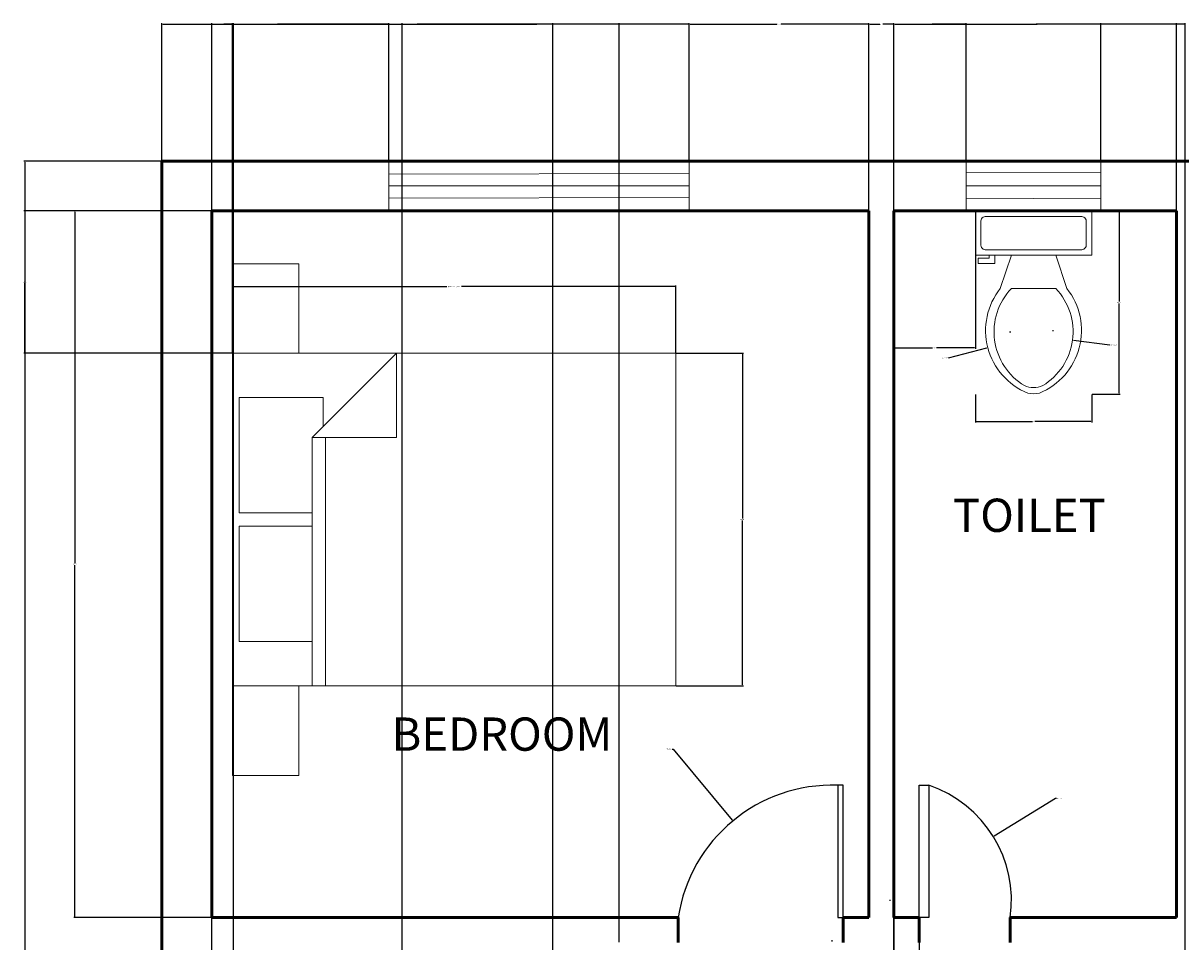
# Model space of a CAD drawing. Units: inches. Extents: x 1926 to 2293, y 1738 to 2280.
# Tile 5 of 6: x 1926 to 2135, y 2114 to 2280. Entities that reach past the tile are written whole.
import ezdxf

# ---------------------------------------------------------------- set-up
doc = ezdxf.new("R2010")
doc.units = ezdxf.units.IN
for name, color, linetype, lineweight in [('A-ANNO-DIMS', 2, 'Continuous', 18), ('A-AREA-IDEN', 7, 'Continuous', 25), ('A-DOOR', 3, 'Continuous', 25), ('A-FLOR-FIXT', 9, 'Continuous', 18), ('A-FURN', 8, 'Continuous', 18), ('A-GLAZ', 4, 'Continuous', 18), ('A-WALL', 7, 'Continuous', 50)]:
    doc.layers.add(name, color=color, linetype=linetype, lineweight=lineweight)
doc.styles.get("Standard").update_dxf_attribs({"font": 'arial.ttf'})
doc.dimstyles.get("Standard").update_dxf_attribs({"dimtxt": 0.18, "dimasz": 0.18, "dimexe": 0.18, "dimexo": 0.0625, "dimgap": 0.09, "dimtad": 0, "dimtih": 1, "dimtoh": 1, "dimdec": 4, "dimzin": 0, "dimdsep": 46, "dimtxsty": 'Standard', "dimcen": 0.09, "dimadec": 0, "dimazin": 0, "dimtfac": 1, "dimtdec": 4, "dimtofl": 0, "dimtmove": 0, "dimatfit": 3, "dimfxl": 1, "dimtolj": 1, "dimtzin": 0, "dimarcsym": 0})

# ---------------------------------------------------------------- blocks, each defined once
blk = doc.blocks.new('Bed - Queen')
for p, q in [((0, -80.00003), (0, 0)), ((0, 0), (59.99999, 0)), ((59.99999, 0), (59.99999, -80.00003)), ((7.99999, -1.2), (28.79998, -1.2)), ((7.99999, -14.4), (7.99999, -1.2)), ((28.79998, -1.2), (28.79998, -14.4)), ((31.19999, -1.2), (51.99999, -1.2)), ((31.19999, -14.4), (31.19999, -1.2)), ((51.99999, -1.2), (51.99999, -16.4)), ((0, -14.4), (44.8, -14.4)), ((59.99999, -29.6), (44.8, -14.4)), ((44.8, -14.4), (44.8, -29.6)), ((51.99999, -16.4), (46.79936, -16.4)), ((44.8, -16.8), (0, -16.8)), ((44.8, -29.6), (59.99999, -29.6)), ((59.99999, -80.00003), (0, -80.00003))]:
    blk.add_line(p, q)
blk = doc.blocks.new('Toilet - top')
for p, q in [((9.5, -6), (9.5, -2)), ((-8, -8.5), (-8, -8)), ((-7, -8), (-7, -9.5)), ((-4, -8), (-6, -14)), ((4, -8), (6, -14)), ((-10, -8.5), (-8, -8.5)), ((-10, -9.5), (-10, -8.5)), ((-7, -9.5), (-10, -9.5)), ((4, -14), (-4, -14))]:
    blk.add_line(p, q)
blk.add_lwpolyline([(10.5, -8), (10.5, 0), (-10.5, 0), (-10.5, -8)], close=True)
for points in [[(-9.5, -2), (-9.5, -6)], [(8.5, -1), (-8.5, -1)], [(-8.5, -7), (8.5, -7)]]:
    blk.add_lwpolyline(points)
for centre, radius, start, end in [((-8.62, -1.88), 0.884, 81.8699, 188.1301), ((8.62, -1.88), 0.884, 351.8699, 98.1301), ((-8.62, -6.12), 0.884, 171.8699, 278.1301), ((8.62, -6.12), 0.884, 261.8699, 8.1301), ((3.52, -21.58), 12.17, 141.4691, 247.9714), ((4.2, -21.82), 11.33, 136.3677, 238.9468), ((-3.52, -21.58), 12.17, 292.0284, 38.5307), ((-4.2, -21.82), 11.33, 301.053, 43.6321), ((0, -27.88), 4, 245.7318, 294.2682), ((0, -29), 4, 254.8605, 285.1395)]:
    blk.add_arc(centre, radius, start, end)
blk = doc.blocks.new('*D6')
at = {"layer": 'A-ANNO-DIMS', "color": 0, "lineweight": -2, "transparency": 16777216}
for p, q in [((1963.48, 2220.56), (1963.48, 2232.68)), ((1963.66, 2232.5), (2002.18, 2232.5)), ((2043.3, 2232.5), (2004.78, 2232.5)), ((2043.48, 2220.56), (2043.48, 2232.68))]:
    blk.add_line(p, q, dxfattribs=at)
at = {"layer": 'A-ANNO-DIMS', "color": 0, "transparency": 16777216}
for points in [[(1963.66, 2232.53), (1963.66, 2232.47), (1963.48, 2232.5)], [(2043.3, 2232.53), (2043.3, 2232.47), (2043.48, 2232.5)]]:
    blk.add_solid(points, dxfattribs=at)
at = {"layer": 'Defpoints', "color": 0, "transparency": 16777216}
for p in [(1963.48, 2232.5), (1963.48, 2220.5), (2043.48, 2220.5)]:
    blk.add_point(p, dxfattribs=at)
at = {"layer": 'A-ANNO-DIMS', "color": 0, "transparency": 16777216, "insert": (2003.48, 2232.5), "char_height": 0.18, "attachment_point": 5}
blk.add_mtext('\\A1;QUEEN BED 80 TYP.', dxfattribs=at)
blk = doc.blocks.new('*D7')
at = {"layer": 'A-ANNO-DIMS', "color": 0, "lineweight": -2, "transparency": 16777216}
for p, q in [((2043.54, 2220.5), (2055.66, 2220.5)), ((2055.48, 2220.32), (2055.48, 2190.68)), ((2055.48, 2160.68), (2055.48, 2190.32)), ((2043.54, 2160.5), (2055.66, 2160.5))]:
    blk.add_line(p, q, dxfattribs=at)
at = {"layer": 'A-ANNO-DIMS', "color": 0, "transparency": 16777216}
for points in [[(2055.45, 2220.32), (2055.51, 2220.32), (2055.48, 2220.5)], [(2055.45, 2160.68), (2055.51, 2160.68), (2055.48, 2160.5)]]:
    blk.add_solid(points, dxfattribs=at)
at = {"layer": 'Defpoints', "color": 0, "transparency": 16777216}
for p in [(2043.48, 2220.5), (2055.48, 2220.5), (2043.48, 2160.5)]:
    blk.add_point(p, dxfattribs=at)
at = {"layer": 'A-ANNO-DIMS', "color": 0, "transparency": 16777216, "insert": (2055.48, 2190.5), "char_height": 0.18, "attachment_point": 5}
blk.add_mtext('\\A1;60 TYP.', dxfattribs=at)
blk = doc.blocks.new('*D14')
at = {"layer": 'A-ANNO-DIMS', "color": 0, "lineweight": -2, "transparency": 16777216}
for p, q in [((2118.53, 2246.16), (2123.6, 2246.16)), ((2123.42, 2245.98), (2123.42, 2229.82)), ((2123.42, 2213.3), (2123.42, 2229.46)), ((2118.53, 2213.12), (2123.6, 2213.12))]:
    blk.add_line(p, q, dxfattribs=at)
at = {"layer": 'A-ANNO-DIMS', "color": 0, "transparency": 16777216}
for points in [[(2123.39, 2245.98), (2123.45, 2245.98), (2123.42, 2246.16)], [(2123.39, 2213.3), (2123.45, 2213.3), (2123.42, 2213.12)]]:
    blk.add_solid(points, dxfattribs=at)
at = {"layer": 'Defpoints', "color": 0, "transparency": 16777216}
for p in [(2118.47, 2246.16), (2123.42, 2246.16), (2118.47, 2213.12)]:
    blk.add_point(p, dxfattribs=at)
at = {"layer": 'A-ANNO-DIMS', "color": 0, "transparency": 16777216, "insert": (2123.42, 2229.64), "char_height": 0.18, "attachment_point": 5}
blk.add_mtext('\\A1;WC 33', dxfattribs=at)
blk = doc.blocks.new('*D15')
at = {"layer": 'A-ANNO-DIMS', "color": 0, "lineweight": -2, "transparency": 16777216}
for p, q in [((2097.47, 2213.05), (2097.47, 2207.98)), ((2118.47, 2213.05), (2118.47, 2207.98)), ((2097.65, 2208.16), (2107.76, 2208.16)), ((2118.29, 2208.16), (2108.17, 2208.16))]:
    blk.add_line(p, q, dxfattribs=at)
at = {"layer": 'A-ANNO-DIMS', "color": 0, "transparency": 16777216}
for points in [[(2097.65, 2208.19), (2097.65, 2208.13), (2097.47, 2208.16)], [(2118.29, 2208.19), (2118.29, 2208.13), (2118.47, 2208.16)]]:
    blk.add_solid(points, dxfattribs=at)
at = {"layer": 'Defpoints', "color": 0, "transparency": 16777216}
for p in [(2097.47, 2213.12), (2118.47, 2213.12), (2118.47, 2208.16)]:
    blk.add_point(p, dxfattribs=at)
at = {"layer": 'A-ANNO-DIMS', "color": 0, "transparency": 16777216, "insert": (2107.97, 2208.16), "char_height": 0.18, "attachment_point": 5}
blk.add_mtext('\\A1;21', dxfattribs=at)
blk = doc.blocks.new('*D16')
at = {"layer": 'A-ANNO-DIMS', "color": 0, "lineweight": -2, "transparency": 16777216}
for p, q in [((1950.76, 2255.22), (1950.76, 2280.04)), ((1950.94, 2279.86), (1970.84, 2279.86)), ((1991.53, 2279.86), (1971.63, 2279.86)), ((1991.71, 2255.22), (1991.71, 2280.04))]:
    blk.add_line(p, q, dxfattribs=at)
at = {"layer": 'A-ANNO-DIMS', "color": 0, "transparency": 16777216}
for points in [[(1950.94, 2279.89), (1950.94, 2279.83), (1950.76, 2279.86)], [(1991.53, 2279.89), (1991.53, 2279.83), (1991.71, 2279.86)]]:
    blk.add_solid(points, dxfattribs=at)
at = {"layer": 'Defpoints', "color": 0, "transparency": 16777216}
for p in [(1991.71, 2279.86), (1950.76, 2255.16), (1991.71, 2255.16)]:
    blk.add_point(p, dxfattribs=at)
at = {"layer": 'A-ANNO-DIMS', "color": 0, "transparency": 16777216, "insert": (1971.24, 2279.86), "char_height": 0.18, "attachment_point": 5}
blk.add_mtext('\\A1;40.96', dxfattribs=at)
blk = doc.blocks.new('*D17')
at = {"layer": 'A-ANNO-DIMS', "color": 0, "lineweight": -2, "transparency": 16777216}
for p, q in [((1991.71, 2255.22), (1991.71, 2280.04)), ((1991.89, 2279.86), (2018.39, 2279.86)), ((2045.68, 2279.86), (2019.18, 2279.86)), ((2045.86, 2255.22), (2045.86, 2280.04))]:
    blk.add_line(p, q, dxfattribs=at)
at = {"layer": 'A-ANNO-DIMS', "color": 0, "transparency": 16777216}
for points in [[(1991.89, 2279.89), (1991.89, 2279.83), (1991.71, 2279.86)], [(2045.68, 2279.89), (2045.68, 2279.83), (2045.86, 2279.86)]]:
    blk.add_solid(points, dxfattribs=at)
at = {"layer": 'Defpoints', "color": 0, "transparency": 16777216}
for p in [(2045.86, 2279.86), (1991.71, 2255.16), (2045.86, 2255.16)]:
    blk.add_point(p, dxfattribs=at)
at = {"layer": 'A-ANNO-DIMS', "color": 0, "transparency": 16777216, "insert": (2018.79, 2279.86), "char_height": 0.18, "attachment_point": 5}
blk.add_mtext('\\A1;54.15', dxfattribs=at)
blk = doc.blocks.new('*D18')
at = {"layer": 'A-ANNO-DIMS', "color": 0, "lineweight": -2, "transparency": 16777216}
for p, q in [((2045.86, 2255.22), (2045.86, 2280.04)), ((2046.04, 2279.86), (2061.67, 2279.86)), ((2078.08, 2279.86), (2062.45, 2279.86)), ((2078.26, 2246.22), (2078.26, 2280.04))]:
    blk.add_line(p, q, dxfattribs=at)
at = {"layer": 'A-ANNO-DIMS', "color": 0, "transparency": 16777216}
for points in [[(2046.04, 2279.89), (2046.04, 2279.83), (2045.86, 2279.86)], [(2078.08, 2279.89), (2078.08, 2279.83), (2078.26, 2279.86)]]:
    blk.add_solid(points, dxfattribs=at)
at = {"layer": 'Defpoints', "color": 0, "transparency": 16777216}
for p in [(2078.26, 2279.86), (2045.86, 2255.16), (2078.26, 2246.16)]:
    blk.add_point(p, dxfattribs=at)
at = {"layer": 'A-ANNO-DIMS', "color": 0, "transparency": 16777216, "insert": (2062.06, 2279.86), "char_height": 0.18, "attachment_point": 5}
blk.add_mtext('\\A1;32.39', dxfattribs=at)
blk = doc.blocks.new('*D19')
at = {"layer": 'A-ANNO-DIMS', "color": 0, "lineweight": -2, "transparency": 16777216}
for p, q in [((2078.26, 2246.22), (2078.26, 2280.04)), ((2078.44, 2279.86), (2080.25, 2279.86)), ((2082.58, 2279.86), (2080.77, 2279.86)), ((2082.76, 2246.22), (2082.76, 2280.04))]:
    blk.add_line(p, q, dxfattribs=at)
at = {"layer": 'A-ANNO-DIMS', "color": 0, "transparency": 16777216}
for points in [[(2078.44, 2279.89), (2078.44, 2279.83), (2078.26, 2279.86)], [(2082.58, 2279.89), (2082.58, 2279.83), (2082.76, 2279.86)]]:
    blk.add_solid(points, dxfattribs=at)
at = {"layer": 'Defpoints', "color": 0, "transparency": 16777216}
for p in [(2082.76, 2279.86), (2078.26, 2246.16), (2082.76, 2246.16)]:
    blk.add_point(p, dxfattribs=at)
at = {"layer": 'A-ANNO-DIMS', "color": 0, "transparency": 16777216, "insert": (2080.51, 2279.86), "char_height": 0.18, "attachment_point": 5}
blk.add_mtext('\\A1;4.5', dxfattribs=at)
blk = doc.blocks.new('*D20')
at = {"layer": 'A-ANNO-DIMS', "color": 0, "lineweight": -2, "transparency": 16777216}
for p, q in [((2082.76, 2246.22), (2082.76, 2280.04)), ((2082.94, 2279.86), (2088.91, 2279.86)), ((2095.66, 2279.86), (2089.68, 2279.86)), ((2095.84, 2255.22), (2095.84, 2280.04))]:
    blk.add_line(p, q, dxfattribs=at)
at = {"layer": 'A-ANNO-DIMS', "color": 0, "transparency": 16777216}
for points in [[(2082.94, 2279.89), (2082.94, 2279.83), (2082.76, 2279.86)], [(2095.66, 2279.89), (2095.66, 2279.83), (2095.84, 2279.86)]]:
    blk.add_solid(points, dxfattribs=at)
at = {"layer": 'Defpoints', "color": 0, "transparency": 16777216}
for p in [(2095.84, 2279.86), (2095.84, 2255.16), (2082.76, 2246.16)]:
    blk.add_point(p, dxfattribs=at)
at = {"layer": 'A-ANNO-DIMS', "color": 0, "transparency": 16777216, "insert": (2089.3, 2279.86), "char_height": 0.18, "attachment_point": 5}
blk.add_mtext('\\A1;13.08', dxfattribs=at)
blk = doc.blocks.new('*D21')
at = {"layer": 'A-ANNO-DIMS', "color": 0, "lineweight": -2, "transparency": 16777216}
for p, q in [((2095.84, 2255.22), (2095.84, 2280.04)), ((2096.02, 2279.86), (2107.5, 2279.86)), ((2119.91, 2279.86), (2108.43, 2279.86)), ((2120.09, 2255.22), (2120.09, 2280.04))]:
    blk.add_line(p, q, dxfattribs=at)
at = {"layer": 'A-ANNO-DIMS', "color": 0, "transparency": 16777216}
for points in [[(2096.02, 2279.89), (2096.02, 2279.83), (2095.84, 2279.86)], [(2119.91, 2279.89), (2119.91, 2279.83), (2120.09, 2279.86)]]:
    blk.add_solid(points, dxfattribs=at)
at = {"layer": 'Defpoints', "color": 0, "transparency": 16777216}
for p in [(2120.09, 2279.86), (2095.84, 2255.16), (2120.09, 2255.16)]:
    blk.add_point(p, dxfattribs=at)
at = {"layer": 'A-ANNO-DIMS', "color": 0, "transparency": 16777216, "insert": (2107.97, 2279.86), "char_height": 0.18, "attachment_point": 5}
blk.add_mtext('\\A1;24.256', dxfattribs=at)
blk = doc.blocks.new('*D22')
at = {"layer": 'A-ANNO-DIMS', "color": 0, "lineweight": -2, "transparency": 16777216}
for p, q in [((2082.76, 2246.22), (2082.76, 2280.04)), ((2082.94, 2279.86), (2108.06, 2279.86)), ((2133.58, 2279.86), (2108.46, 2279.86)), ((2133.76, 2246.22), (2133.76, 2280.04))]:
    blk.add_line(p, q, dxfattribs=at)
at = {"layer": 'A-ANNO-DIMS', "color": 0, "transparency": 16777216}
for points in [[(2082.94, 2279.89), (2082.94, 2279.83), (2082.76, 2279.86)], [(2133.58, 2279.89), (2133.58, 2279.83), (2133.76, 2279.86)]]:
    blk.add_solid(points, dxfattribs=at)
at = {"layer": 'Defpoints', "color": 0, "transparency": 16777216}
for p in [(2133.76, 2279.86), (2082.76, 2246.16), (2133.76, 2246.16)]:
    blk.add_point(p, dxfattribs=at)
at = {"layer": 'A-ANNO-DIMS', "color": 0, "transparency": 16777216, "insert": (2108.26, 2279.86), "char_height": 0.18, "attachment_point": 5}
blk.add_mtext('\\A1;51', dxfattribs=at)
blk = doc.blocks.new('*D41')
at = {"layer": 'A-ANNO-DIMS', "color": 0, "lineweight": -2, "transparency": 16777216}
for p, q in [((1959.69, 2246.16), (1934.88, 2246.16)), ((1935.06, 2245.98), (1935.06, 2182.59)), ((1935.06, 2118.84), (1935.06, 2182.23)), ((1959.69, 2118.66), (1934.88, 2118.66))]:
    blk.add_line(p, q, dxfattribs=at)
at = {"layer": 'A-ANNO-DIMS', "color": 0, "transparency": 16777216}
for points in [[(1935.03, 2245.98), (1935.09, 2245.98), (1935.06, 2246.16)], [(1935.03, 2118.84), (1935.09, 2118.84), (1935.06, 2118.66)]]:
    blk.add_solid(points, dxfattribs=at)
at = {"layer": 'Defpoints', "color": 0, "transparency": 16777216}
for p in [(1935.06, 2246.16), (1959.76, 2246.16), (1959.76, 2118.66)]:
    blk.add_point(p, dxfattribs=at)
at = {"layer": 'A-ANNO-DIMS', "color": 0, "transparency": 16777216, "insert": (1935.06, 2182.41), "char_height": 0.18, "attachment_point": 5}
blk.add_mtext('\\A1;127.5', dxfattribs=at)
blk = doc.blocks.new('*D46')
at = {"layer": 'A-ANNO-DIMS', "color": 0, "lineweight": -2, "transparency": 16777216}
for p, q in [((1959.76, 2114.22), (1959.76, 2280.04)), ((1959.94, 2279.86), (1996.18, 2279.86)), ((2033.08, 2279.86), (1996.83, 2279.86)), ((2033.26, 2114.22), (2033.26, 2280.04))]:
    blk.add_line(p, q, dxfattribs=at)
at = {"layer": 'A-ANNO-DIMS', "color": 0, "transparency": 16777216}
for points in [[(1959.94, 2279.89), (1959.94, 2279.83), (1959.76, 2279.86)], [(2033.08, 2279.89), (2033.08, 2279.83), (2033.26, 2279.86)]]:
    blk.add_solid(points, dxfattribs=at)
at = {"layer": 'Defpoints', "color": 0, "transparency": 16777216}
for p in [(2033.26, 2279.86), (1959.76, 2114.16), (2033.26, 2114.16)]:
    blk.add_point(p, dxfattribs=at)
at = {"layer": 'A-ANNO-DIMS', "color": 0, "transparency": 16777216, "insert": (1996.51, 2279.86), "char_height": 0.18, "attachment_point": 5}
blk.add_mtext('\\A1;73.5', dxfattribs=at)
blk = doc.blocks.new('*D53')
at = {"layer": 'A-ANNO-DIMS', "color": 0, "lineweight": -2, "transparency": 16777216}
for p, q in [((1994.13, 2111.62), (1994.13, 2280.04)), ((1994.31, 2279.86), (2007.3, 2279.86)), ((2021.07, 2279.86), (2008.09, 2279.86)), ((2021.25, 2111.62), (2021.25, 2280.04))]:
    blk.add_line(p, q, dxfattribs=at)
at = {"layer": 'A-ANNO-DIMS', "color": 0, "transparency": 16777216}
for points in [[(1994.31, 2279.89), (1994.31, 2279.83), (1994.13, 2279.86)], [(2021.07, 2279.89), (2021.07, 2279.83), (2021.25, 2279.86)]]:
    blk.add_solid(points, dxfattribs=at)
at = {"layer": 'Defpoints', "color": 0, "transparency": 16777216}
for p in [(2021.25, 2279.86), (1994.13, 2111.56), (2021.25, 2111.56)]:
    blk.add_point(p, dxfattribs=at)
at = {"layer": 'A-ANNO-DIMS', "color": 0, "transparency": 16777216, "insert": (2007.69, 2279.86), "char_height": 0.18, "attachment_point": 5}
blk.add_mtext('\\A1;27.13', dxfattribs=at)
blk = doc.blocks.new('*D59')
at = {"layer": 'A-ANNO-DIMS', "color": 0, "lineweight": -2, "transparency": 16777216}
for p, q in [((2082.76, 2118.6), (2082.76, 2093.78)), ((2087.35, 2118.6), (2087.35, 2093.78)), ((2082.94, 2093.96), (2084.66, 2093.96)), ((2087.17, 2093.96), (2085.45, 2093.96))]:
    blk.add_line(p, q, dxfattribs=at)
at = {"layer": 'A-ANNO-DIMS', "color": 0, "transparency": 16777216}
for points in [[(2082.94, 2093.99), (2082.94, 2093.93), (2082.76, 2093.96)], [(2087.17, 2093.99), (2087.17, 2093.93), (2087.35, 2093.96)]]:
    blk.add_solid(points, dxfattribs=at)
at = {"layer": 'Defpoints', "color": 0, "transparency": 16777216}
for p in [(2082.76, 2118.66), (2087.35, 2118.66), (2082.76, 2093.96)]:
    blk.add_point(p, dxfattribs=at)
at = {"layer": 'A-ANNO-DIMS', "color": 0, "transparency": 16777216, "insert": (2085.05, 2093.96), "char_height": 0.18, "attachment_point": 5}
blk.add_mtext('\\A1;4.595', dxfattribs=at)
blk = doc.blocks.new('*D61')
at = {"layer": 'A-ANNO-DIMS', "color": 0, "lineweight": -2, "transparency": 16777216}
for p, q in [((2082.76, 1933.22), (2082.76, 2280.04)), ((2082.94, 2279.86), (2108.63, 2279.86)), ((2135.12, 2279.86), (2109.42, 2279.86)), ((2135.3, 1933.22), (2135.3, 2280.04))]:
    blk.add_line(p, q, dxfattribs=at)
at = {"layer": 'A-ANNO-DIMS', "color": 0, "transparency": 16777216}
for points in [[(2082.94, 2279.89), (2082.94, 2279.83), (2082.76, 2279.86)], [(2135.12, 2279.89), (2135.12, 2279.83), (2135.3, 2279.86)]]:
    blk.add_solid(points, dxfattribs=at)
at = {"layer": 'Defpoints', "color": 0, "transparency": 16777216}
for p in [(2135.3, 2279.86), (2082.76, 1933.16), (2135.3, 1933.16)]:
    blk.add_point(p, dxfattribs=at)
at = {"layer": 'A-ANNO-DIMS', "color": 0, "transparency": 16777216, "insert": (2109.03, 2279.86), "char_height": 0.18, "attachment_point": 5}
blk.add_mtext('\\A1;52.54', dxfattribs=at)
blk = doc.blocks.new('*D75')
at = {"layer": 'A-ANNO-DIMS', "color": 0, "lineweight": -2, "transparency": 16777216}
for p, q in [((1959.76, 2246.22), (1959.76, 2280.04)), ((1959.94, 2279.86), (1961.29, 2279.86)), ((1963.3, 2279.86), (1961.94, 2279.86)), ((1963.48, 2220.56), (1963.48, 2280.04))]:
    blk.add_line(p, q, dxfattribs=at)
at = {"layer": 'A-ANNO-DIMS', "color": 0, "transparency": 16777216}
for points in [[(1959.94, 2279.89), (1959.94, 2279.83), (1959.76, 2279.86)], [(1963.3, 2279.89), (1963.3, 2279.83), (1963.48, 2279.86)]]:
    blk.add_solid(points, dxfattribs=at)
at = {"layer": 'Defpoints', "color": 0, "transparency": 16777216}
for p in [(1959.76, 2279.86), (1959.76, 2246.16), (1963.48, 2220.5)]:
    blk.add_point(p, dxfattribs=at)
at = {"layer": 'A-ANNO-DIMS', "color": 0, "transparency": 16777216, "insert": (1961.62, 2279.86), "char_height": 0.18, "attachment_point": 5}
blk.add_mtext('\\A1;3.72', dxfattribs=at)
blk = doc.blocks.new('*D76')
at = {"layer": 'A-ANNO-DIMS', "color": 0, "lineweight": -2, "transparency": 16777216}
for p, q in [((1959.69, 2246.16), (1925.88, 2246.16)), ((1926.06, 2245.98), (1926.06, 2233.51)), ((1926.06, 2220.68), (1926.06, 2233.15)), ((1963.42, 2220.5), (1925.88, 2220.5))]:
    blk.add_line(p, q, dxfattribs=at)
at = {"layer": 'A-ANNO-DIMS', "color": 0, "transparency": 16777216}
for points in [[(1926.03, 2245.98), (1926.09, 2245.98), (1926.06, 2246.16)], [(1926.03, 2220.68), (1926.09, 2220.68), (1926.06, 2220.5)]]:
    blk.add_solid(points, dxfattribs=at)
at = {"layer": 'Defpoints', "color": 0, "transparency": 16777216}
for p in [(1926.06, 2246.16), (1959.76, 2246.16), (1963.48, 2220.5)]:
    blk.add_point(p, dxfattribs=at)
at = {"layer": 'A-ANNO-DIMS', "color": 0, "transparency": 16777216, "insert": (1926.06, 2233.33), "char_height": 0.18, "attachment_point": 5}
blk.add_mtext('\\A1;25.66', dxfattribs=at)
blk = doc.blocks.new('*D79')
at = {"layer": 'A-ANNO-DIMS', "color": 0, "lineweight": -2, "transparency": 16777216}
for p, q in [((1959.76, 1833.35), (1959.76, 2280.04)), ((1959.94, 2279.86), (1961.41, 2279.86)), ((1963.53, 2279.86), (1962.06, 2279.86)), ((1963.71, 1828.81), (1963.71, 2280.04))]:
    blk.add_line(p, q, dxfattribs=at)
at = {"layer": 'A-ANNO-DIMS', "color": 0, "transparency": 16777216}
for points in [[(1959.94, 2279.89), (1959.94, 2279.83), (1959.76, 2279.86)], [(1963.53, 2279.89), (1963.53, 2279.83), (1963.71, 2279.86)]]:
    blk.add_solid(points, dxfattribs=at)
at = {"layer": 'Defpoints', "color": 0, "transparency": 16777216}
for p in [(1959.76, 2279.86), (1959.76, 1833.29), (1963.71, 1828.75)]:
    blk.add_point(p, dxfattribs=at)
at = {"layer": 'A-ANNO-DIMS', "color": 0, "transparency": 16777216, "insert": (1961.74, 2279.86), "char_height": 0.18, "attachment_point": 5}
blk.add_mtext('\\A1;3.96', dxfattribs=at)
blk = doc.blocks.new('*D83')
at = {"layer": 'A-ANNO-DIMS', "color": 0, "lineweight": -2, "transparency": 16777216}
for p, q in [((2082.76, 2246.1), (2082.76, 2221.28)), ((2097.47, 2246.1), (2097.47, 2221.28)), ((2082.94, 2221.46), (2089.74, 2221.46)), ((2097.29, 2221.46), (2090.48, 2221.46))]:
    blk.add_line(p, q, dxfattribs=at)
at = {"layer": 'A-ANNO-DIMS', "color": 0, "transparency": 16777216}
for points in [[(2082.94, 2221.49), (2082.94, 2221.43), (2082.76, 2221.46)], [(2097.29, 2221.49), (2097.29, 2221.43), (2097.47, 2221.46)]]:
    blk.add_solid(points, dxfattribs=at)
at = {"layer": 'Defpoints', "color": 0, "transparency": 16777216}
for p in [(2082.76, 2246.16), (2097.47, 2246.16), (2082.76, 2221.46)]:
    blk.add_point(p, dxfattribs=at)
at = {"layer": 'A-ANNO-DIMS', "color": 0, "transparency": 16777216, "insert": (2090.11, 2221.46), "char_height": 0.18, "attachment_point": 5}
blk.add_mtext('\\A1;14.71', dxfattribs=at)
blk = doc.blocks.new('*D85')
at = {"layer": 'A-ANNO-DIMS', "color": 0, "lineweight": -2, "transparency": 16777216}
for p, q in [((1950.69, 2255.16), (1925.88, 2255.16)), ((1926.06, 2254.98), (1926.06, 2024.34)), ((1926.06, 1793.34), (1926.06, 2023.98)), ((1950.69, 1793.16), (1925.88, 1793.16))]:
    blk.add_line(p, q, dxfattribs=at)
at = {"layer": 'A-ANNO-DIMS', "color": 0, "transparency": 16777216}
for points in [[(1926.03, 2254.98), (1926.09, 2254.98), (1926.06, 2255.16)], [(1926.03, 1793.34), (1926.09, 1793.34), (1926.06, 1793.16)]]:
    blk.add_solid(points, dxfattribs=at)
at = {"layer": 'Defpoints', "color": 0, "transparency": 16777216}
for p in [(1926.06, 2255.16), (1950.76, 2255.16), (1950.76, 1793.16)]:
    blk.add_point(p, dxfattribs=at)
at = {"layer": 'A-ANNO-DIMS', "color": 0, "transparency": 16777216, "insert": (1926.06, 2024.16), "char_height": 0.18, "attachment_point": 5}
blk.add_mtext('\\A1;462', dxfattribs=at)
blk = doc.blocks.new('*D90')
at = {"layer": 'A-ANNO-DIMS', "color": 0, "lineweight": -2, "transparency": 16777216}
for p, q in [((2042.78, 2149.04), (2042.96, 2149.04)), ((2042.96, 2149.04), (2053.59, 2136.23)), ((2071.53, 2114.5), (2071.71, 2114.5)), ((2071.62, 2114.41), (2071.62, 2114.59))]:
    blk.add_line(p, q, dxfattribs=at)
at = {"layer": 'A-ANNO-DIMS', "color": 0, "transparency": 16777216}
blk.add_solid([(2053.61, 2136.25), (2053.57, 2136.21), (2053.71, 2136.09)], dxfattribs=at)
at = {"layer": 'Defpoints', "color": 0, "transparency": 16777216}
for p in [(2053.71, 2136.09), (2071.62, 2114.5)]:
    blk.add_point(p, dxfattribs=at)
at = {"layer": 'A-ANNO-DIMS', "color": 0, "transparency": 16777216, "insert": (2042.23, 2149.04), "char_height": 0.18, "attachment_point": 5}
blk.add_mtext('\\A1;R28.053', dxfattribs=at)
blk = doc.blocks.new('*D92')
at = {"layer": 'A-ANNO-DIMS', "color": 0, "lineweight": -2, "transparency": 16777216}
for p, q in [((2111.92, 2140.15), (2100.88, 2133.36)), ((2112.1, 2140.15), (2111.92, 2140.15)), ((2081.99, 2121.78), (2082.17, 2121.78)), ((2082.08, 2121.69), (2082.08, 2121.87))]:
    blk.add_line(p, q, dxfattribs=at)
at = {"layer": 'A-ANNO-DIMS', "color": 0, "transparency": 16777216}
blk.add_solid([(2100.87, 2133.38), (2100.9, 2133.33), (2100.73, 2133.26)], dxfattribs=at)
at = {"layer": 'Defpoints', "color": 0, "transparency": 16777216}
for p in [(2100.73, 2133.26), (2082.08, 2121.78)]:
    blk.add_point(p, dxfattribs=at)
at = {"layer": 'A-ANNO-DIMS', "color": 0, "transparency": 16777216, "insert": (2112.65, 2140.15), "char_height": 0.18, "attachment_point": 5}
blk.add_mtext('\\A1;R21.897', dxfattribs=at)
blk = doc.blocks.new('*D107')
at = {"layer": 'A-ANNO-DIMS', "color": 0, "lineweight": -2, "transparency": 16777216}
for p, q in [((2111.4, 2224.58), (2111.58, 2224.58)), ((2111.49, 2224.49), (2111.49, 2224.67)), ((2092.65, 2219.63), (2099.54, 2221.44))]:
    blk.add_line(p, q, dxfattribs=at)
at = {"layer": 'A-ANNO-DIMS', "color": 0, "transparency": 16777216}
blk.add_solid([(2099.53, 2221.47), (2099.55, 2221.42), (2099.72, 2221.49)], dxfattribs=at)
at = {"layer": 'Defpoints', "color": 0, "transparency": 16777216}
for p in [(2111.49, 2224.58), (2099.72, 2221.49)]:
    blk.add_point(p, dxfattribs=at)
at = {"layer": 'A-ANNO-DIMS', "color": 0, "transparency": 16777216, "insert": (2091.98, 2219.63), "char_height": 0.18, "attachment_point": 5}
blk.add_mtext('\\A1;2X R12.17', dxfattribs=at)
blk = doc.blocks.new('*D108')
at = {"layer": 'A-ANNO-DIMS', "color": 0, "lineweight": -2, "transparency": 16777216}
for p, q in [((2103.68, 2224.34), (2103.86, 2224.34)), ((2103.77, 2224.25), (2103.77, 2224.43)), ((2121.73, 2221.93), (2115.17, 2222.81))]:
    blk.add_line(p, q, dxfattribs=at)
at = {"layer": 'A-ANNO-DIMS', "color": 0, "transparency": 16777216}
blk.add_solid([(2115.18, 2222.84), (2115.17, 2222.78), (2114.99, 2222.83)], dxfattribs=at)
at = {"layer": 'Defpoints', "color": 0, "transparency": 16777216}
for p in [(2103.77, 2224.34), (2114.99, 2222.83)]:
    blk.add_point(p, dxfattribs=at)
at = {"layer": 'A-ANNO-DIMS', "color": 0, "transparency": 16777216, "insert": (2122.41, 2221.93), "char_height": 0.18, "attachment_point": 5}
blk.add_mtext('\\A1;2X R11.33', dxfattribs=at)

msp = doc.modelspace()

# ---------------------------------------------------------------- linework, layer by layer
at = {"layer": 'A-DOOR'}
for p, q in [((2072.6476, 2142.5375), (2072.6476, 2118.6622)), ((2073.6065, 2142.5375), (2072.6476, 2142.5375)), ((2073.6065, 2118.6622), (2073.6065, 2142.5375)), ((2087.3518, 2118.6622), (2087.3518, 2142.5375)), ((2087.3518, 2142.5375), (2089.0597, 2142.5375)), ((2089.0597, 2142.5375), (2089.0597, 2118.6622)), ((2072.6476, 2118.6622), (2073.6065, 2118.6622)), ((2089.0597, 2118.6622), (2087.3518, 2118.6622))]:
    msp.add_line(p, q, dxfattribs=at)
for centre, radius, start, end in [((2071.6208, 2114.5028), 28.0535, 87.90233, 171.473485), ((2082.0837, 2121.7819), 21.8965, 351.808921, 71.422384)]:
    msp.add_arc(centre, radius, start, end, dxfattribs=at)
at = {"layer": 'A-FURN'}
for points in [[(1963.4784, 2220.5005), (1975.4784, 2220.5005), (1975.4784, 2236.6188), (1963.4784, 2236.6188)], [(1963.4784, 2160.5005), (1975.4784, 2160.5005), (1975.4784, 2144.2897), (1963.4784, 2144.2897)]]:
    msp.add_lwpolyline(points, close=True, dxfattribs=at)
at = {"layer": 'A-GLAZ'}
for p, q in [((1991.7142, 2252.7963), (2045.8637, 2252.9154)), ((2095.838, 2253.0985), (2120.0938, 2253.0246)), ((1991.7142, 2250.6622), (2045.8637, 2250.6622)), ((2095.838, 2250.6622), (2120.0938, 2250.6622)), ((1991.7142, 2248.4517), (2045.8637, 2248.5707)), ((2095.838, 2248.3298), (2120.0938, 2248.4776))]:
    msp.add_line(p, q, dxfattribs=at)
for points in [[(1991.7142, 2255.1622), (2045.8637, 2255.1622), (2045.8637, 2246.1622), (1991.7142, 2246.1622)], [(2095.838, 2255.1622), (2120.0938, 2255.1622), (2120.0938, 2246.1622), (2095.838, 2246.1622)]]:
    msp.add_lwpolyline(points, close=True, dxfattribs=at)
at = {"layer": 'A-WALL'}
for p, q in [((1950.7569, 2255.1622), (2256.7569, 2255.1622)), ((1950.7569, 1793.1622), (1950.7569, 2255.1622)), ((1959.7569, 2246.1622), (2078.2569, 2246.1622)), ((1959.7569, 2118.6622), (1959.7569, 2246.1622)), ((2078.2569, 2246.1622), (2078.2569, 2118.6622)), ((2082.7569, 2246.1622), (2082.7569, 2118.6622)), ((2082.7569, 2246.1622), (2082.7569, 2118.6622)), ((2082.7569, 2246.1622), (2133.7569, 2246.1622)), ((2133.7569, 2118.6622), (2133.7569, 2246.1622)), ((1959.7569, 2118.6622), (2043.8774, 2118.6622)), ((2043.8774, 2114.1622), (2043.8774, 2118.6622)), ((2073.6065, 2114.1622), (2073.6065, 2118.6622)), ((2073.6065, 2118.6622), (2078.2569, 2118.6622)), ((2082.7569, 2118.6622), (2087.3518, 2118.6622)), ((2087.3518, 2114.1622), (2087.3518, 2118.6622)), ((2103.7569, 2114.1622), (2103.7569, 2118.6622)), ((2103.7569, 2118.6622), (2133.7569, 2118.6622))]:
    msp.add_line(p, q, dxfattribs=at)

# ---------------------------------------------------------------- block references
at = {"layer": 'A-FLOR-FIXT'}
msp.add_blockref('Toilet - top', (2107.9659, 2246.1622), dxfattribs=at)
at = {"layer": 'A-FURN', "rotation": 90}
msp.add_blockref('Bed - Queen', (1963.4784, 2160.5005), dxfattribs=at)

# ---------------------------------------------------------------- texts
at = {"layer": 'A-AREA-IDEN', "char_height": 6, "attachment_point": 1}
for s, insert in [('TOILET', (2093.4402, 2194.251)), ('BEDROOM', (1992.1816, 2154.7681))]:
    msp.add_mtext_dynamic_manual_height_columns(s, width=23.953264, gutter_width=12.5, heights=[0], dxfattribs=dict(at, insert=insert))

# ---------------------------------------------------------------- dimensions: what is measured, and where the dimension line sits
at = {"layer": 'A-ANNO-DIMS'}
for base, p1, p2, override, picture, middle in [((1991.7142, 2279.8622), (1950.7569, 2255.1622), (1991.7142, 2255.1622), {"dimdec": 2, "dimlfac": 1, "dimrnd": 0, "dimzin": 0, "dimdsep": 46, "dimlunit": 2}, '*D16', (1971.2355, 2279.8622)), ((2033.2569, 2279.8622), (1959.7569, 2114.1622), (2033.2569, 2114.1622), {"dimdec": 1, "dimlfac": 1, "dimrnd": 0, "dimzin": 0, "dimdsep": 46, "dimlunit": 2}, '*D46', (1996.5069, 2279.8622)), ((1959.7569, 2279.8622), (1963.4784, 2220.5005), (1959.7569, 2246.1622), {"dimdec": 2, "dimlfac": 1, "dimrnd": 0, "dimzin": 0, "dimdsep": 46, "dimlunit": 2}, '*D75', (1961.6176, 2279.8622)), ((1959.7569, 2279.8622), (1963.7133, 1828.7469), (1959.7569, 1833.2892), {"dimdec": 2, "dimlfac": 1, "dimrnd": 0, "dimzin": 0, "dimdsep": 46, "dimlunit": 2}, '*D79', (1961.7351, 2279.8622)), ((2045.8637, 2279.8622), (1991.7142, 2255.1622), (2045.8637, 2255.1622), {"dimdec": 2, "dimlfac": 1, "dimrnd": 0, "dimzin": 0, "dimdsep": 46, "dimlunit": 2}, '*D17', (2018.789, 2279.8622)), ((2021.2546, 2279.8622), (1994.1266, 2111.5596), (2021.2546, 2111.5596), {"dimdec": 2, "dimlfac": 1, "dimrnd": 0, "dimzin": 0, "dimdsep": 46, "dimlunit": 2}, '*D53', (2007.6906, 2279.8622)), ((2078.2569, 2279.8622), (2045.8637, 2255.1622), (2078.2569, 2246.1622), {"dimdec": 2, "dimlfac": 1, "dimrnd": 0, "dimzin": 0, "dimdsep": 46, "dimlunit": 2}, '*D18', (2062.0603, 2279.8622)), ((2082.7569, 2279.8622), (2078.2569, 2246.1622), (2082.7569, 2246.1622), {"dimdec": 1, "dimlfac": 1, "dimrnd": 0, "dimzin": 0, "dimdsep": 46, "dimlunit": 2}, '*D19', (2080.5069, 2279.8622)), ((2095.838, 2279.8622), (2082.7569, 2246.1622), (2095.838, 2255.1622), {"dimdec": 2, "dimlfac": 1, "dimrnd": 0, "dimzin": 0, "dimdsep": 46, "dimlunit": 2}, '*D20', (2089.2974, 2279.8622)), ((2133.7569, 2279.8622), (2082.7569, 2246.1622), (2133.7569, 2246.1622), {"dimdec": 0, "dimlfac": 1, "dimrnd": 0, "dimzin": 0, "dimdsep": 46, "dimlunit": 2}, '*D22', (2108.2569, 2279.8622)), ((2135.2979, 2279.8622), (2082.7569, 1933.1622), (2135.2979, 1933.1622), {"dimdec": 2, "dimlfac": 1, "dimrnd": 0, "dimzin": 0, "dimdsep": 46, "dimlunit": 2}, '*D61', (2109.0274, 2279.8622)), ((2120.0938, 2279.8622), (2095.838, 2255.1622), (2120.0938, 2255.1622), {"dimdec": 3, "dimlfac": 1, "dimrnd": 0, "dimzin": 0, "dimdsep": 46, "dimlunit": 2}, '*D21', (2107.9659, 2279.8622)), ((2118.4659, 2208.159), (2097.4659, 2213.116), (2118.4659, 2213.116), {"dimdec": 0, "dimlfac": 1, "dimrnd": 0, "dimzin": 0, "dimdsep": 46, "dimlunit": 2}, '*D15', (2107.9659, 2208.159))]:
    dim = msp.add_linear_dim(base=base, p1=p1, p2=p2, dimstyle='Standard', override=override, dxfattribs=at)
    dim.commit()
    dim.dimension.update_dxf_attribs({"geometry": picture, "text_midpoint": middle})
for base, p1, p2, angle, override, picture, middle in [((1926.0569, 2255.1622), (1950.7569, 1793.1622), (1950.7569, 2255.1622), 90, {"dimdec": 0, "dimlfac": 1, "dimrnd": 0, "dimzin": 0, "dimdsep": 46, "dimlunit": 2}, '*D85', (1926.0569, 2024.1622)), ((1926.0569, 2246.1622), (1963.4784, 2220.5005), (1959.7569, 2246.1622), 90, {"dimdec": 2, "dimlfac": 1, "dimrnd": 0, "dimzin": 0, "dimdsep": 46, "dimlunit": 2}, '*D76', (1926.0569, 2233.3314)), ((1935.0569, 2246.1622), (1959.7569, 2118.6622), (1959.7569, 2246.1622), 90, {"dimdec": 1, "dimlfac": 1, "dimrnd": 0, "dimzin": 0, "dimdsep": 46, "dimlunit": 2}, '*D41', (1935.0569, 2182.4122)), ((2082.7569, 2221.4622), (2097.4659, 2246.1622), (2082.7569, 2246.1622), 180, {"dimdec": 2, "dimlfac": 1, "dimrnd": 0, "dimzin": 0, "dimdsep": 46, "dimlunit": 2}, '*D83', (2090.1114, 2221.4622)), ((2082.7569, 2093.9622), (2087.3518, 2118.6622), (2082.7569, 2118.6622), 180, {"dimdec": 3, "dimlfac": 1, "dimrnd": 0, "dimzin": 0, "dimdsep": 46, "dimlunit": 2}, '*D59', (2085.0543, 2093.9622))]:
    dim = msp.add_linear_dim(base=base, p1=p1, p2=p2, angle=angle, dimstyle='Standard', override=override, dxfattribs=at)
    dim.commit()
    dim.dimension.update_dxf_attribs({"geometry": picture, "text_midpoint": middle})
for base, p1, p2, angle, text, picture, middle in [((2123.4228, 2246.1622), (2118.4659, 2213.116), (2118.4659, 2246.1622), 90, 'WC <>', '*D14', (2123.4228, 2229.6391)), ((1963.4784, 2232.5005), (2043.4784, 2220.5005), (1963.4784, 2220.5005), 180, 'QUEEN BED <> TYP.', '*D6', (2003.4784, 2232.5005)), ((2055.4784, 2220.5005), (2043.4784, 2160.5005), (2043.4784, 2220.5005), 90, '<> TYP.', '*D7', (2055.4784, 2190.5005))]:
    dim = msp.add_linear_dim(base=base, p1=p1, p2=p2, angle=angle, text=text, dimstyle='Standard', override={"dimdec": 0, "dimlfac": 1, "dimrnd": 0, "dimzin": 0, "dimdsep": 46, "dimlunit": 2}, dxfattribs=at)
    dim.commit()
    dim.dimension.update_dxf_attribs({"geometry": picture, "text_midpoint": middle})
for center, mpoint, picture, middle in [((2111.4855, 2224.5817), (2099.7158, 2221.4899), '*D107', (2092.6539, 2219.6349)), ((2103.766, 2224.3448), (2114.9941, 2222.835), '*D108', (2121.731, 2221.9291))]:
    dim = msp.add_radius_dim(center=center, mpoint=mpoint, text='2X <>', dimstyle='Standard', override={"dimdec": 2, "dimlfac": 1, "dimrnd": 0, "dimzin": 0, "dimdsep": 46, "dimlunit": 2}, dxfattribs=at)
    dim.commit()
    dim.dimension.update_dxf_attribs({"geometry": picture, "text_midpoint": middle, "dimtype": 164})
for center, mpoint, picture, middle in [((2071.6208, 2114.5028), (2053.7059, 2136.0911), '*D90', (2042.2272, 2149.0441)), ((2082.0837, 2121.7819), (2100.7301, 2133.2611), '*D92', (2112.6477, 2140.1485))]:
    dim = msp.add_radius_dim(center=center, mpoint=mpoint, dimstyle='Standard', override={"dimdec": 3, "dimlfac": 1, "dimrnd": 0, "dimzin": 0, "dimdsep": 46, "dimlunit": 2}, dxfattribs=at)
    dim.commit()
    dim.dimension.update_dxf_attribs({"geometry": picture, "text_midpoint": middle, "dimtype": 164})

doc.saveas('drawing.dxf')
